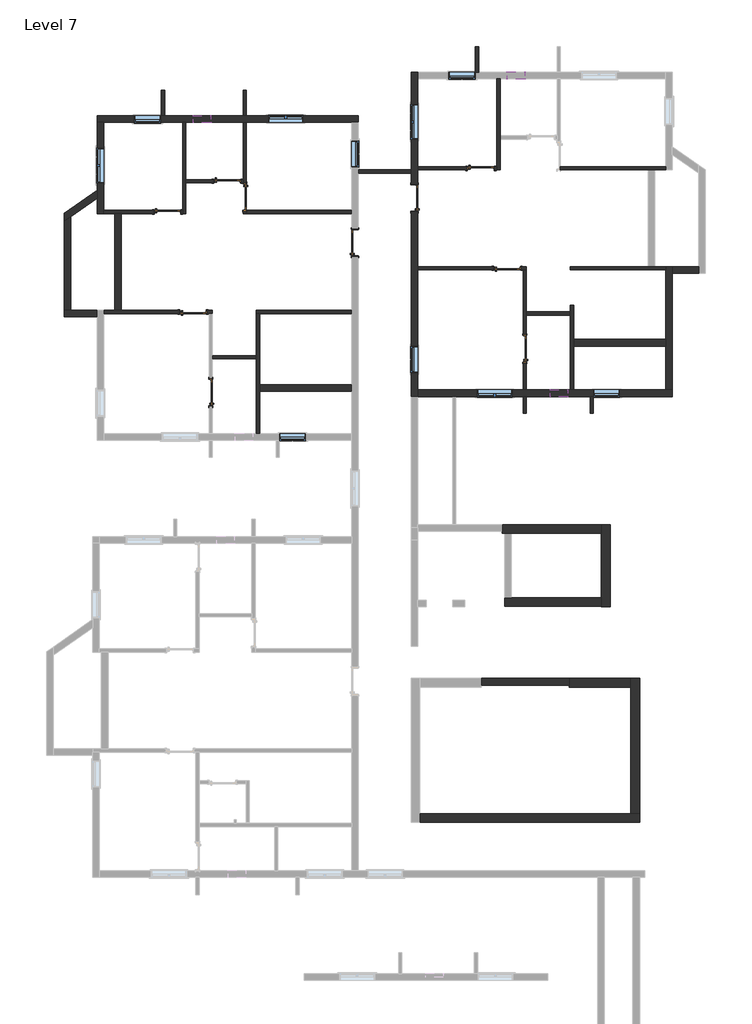
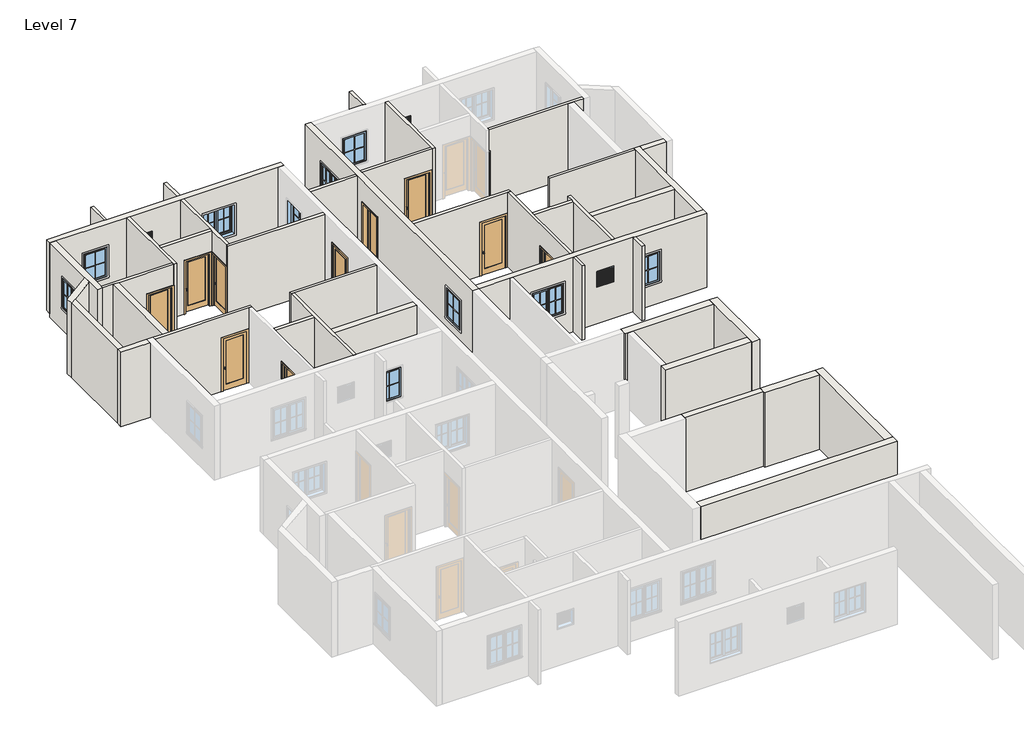
# One storey, part 5 of 7: 42 walls, 13 windows, 10 doors.
"""IFC4 building model written with IfcOpenShell, lengths in millimetres."""

from ifc_helpers import new_model, si_unit, frame, origin, place, context, project, spatial, polyline, outline, extrude, faceted_brep, transform, mapped, element, save
from components import door_3c6ab76a, door_a3feeac7, door_3b97b8e7, door_868ee8a9, window_272f20d6, window_casement_double_4_x_4_af3140d2, window_f2d8fef0

model = new_model("IFC4")

# Units and contexts
model_context = context("Model", 3, world=origin())
ifc_project = project(units=[si_unit("LENGTHUNIT", "METRE", prefix="MILLI")], contexts=[model_context])

# Site, building, storey
site = spatial("IfcSite", under=ifc_project)
building = spatial("IfcBuilding", under=site)
storey = spatial("IfcBuildingStorey", under=building, Name="Level 7", Elevation=9601.2)

# Doors
placement = place(None, origin())
door_shape = door_3c6ab76a(model_context)
element("IfcDoor", 1, ObjectType="Door-Interior-Single-1_Panel-Wood : 2'6\" x 7' door", at=placement, inside=storey, context=model_context, shape_type="MappedRepresentation", body=[
    mapped(door_shape, transform((-10226.9509469, 25492.3711172, 9601.2), x_axis=(1.0, 0.0, 0.0), y_axis=(0.0, 1.0, 0.0), z_axis=(0.0, 0.0, 1.0))),
])
door_2_shape = door_a3feeac7(model_context)
element("IfcDoor", 2, ObjectType="Door-Interior-Single-1_Panel-Wood : 2'6\" x 7' door", at=placement, inside=storey, context=model_context, shape_type="MappedRepresentation", body=[
    mapped(door_2_shape, transform((-10795.2759469, 18161.2961172, 9601.2), x_axis=(0.0, 1.0, 0.0), y_axis=(-1.0, 0.0, 0.0), z_axis=(0.0, 0.0, 1.0))),
])
element("IfcDoor", 3, ObjectType="Door-Interior-Single-1_Panel-Wood : 2'6\" x 7' door", at=placement, inside=storey, context=model_context, shape_type="MappedRepresentation", body=[
    mapped(door_2_shape, transform((101.3240531, 19674.7755084, 9601.2), x_axis=(0.0, 1.0, 0.0), y_axis=(-1.0, 0.0, 0.0), z_axis=(0.0, 0.0, 1.0))),
])
element("IfcDoor", 4, ObjectType="Door-Interior-Single-1_Panel-Wood : 36\" x 84\"", at=placement, inside=storey, context=model_context, shape_type="MappedRepresentation", body=[
    mapped(door_shape, transform((-12297.0509469, 24425.5711172, 9601.2), x_axis=(1.0, 0.0, 0.0), y_axis=(0.0, 1.0, 0.0), z_axis=(0.0, 0.0, 1.0))),
])
element("IfcDoor", 5, ObjectType="Door-Interior-Single-1_Panel-Wood : 36\" x 84\"", at=placement, inside=storey, context=model_context, shape_type="MappedRepresentation", body=[
    mapped(door_shape, transform((-9614.1759469, 24936.7461172, 9601.2), x_axis=(0.0, -1.0, 0.0), y_axis=(1.0, 0.0, 0.0), z_axis=(0.0, 0.0, 1.0))),
])
element("IfcDoor", 6, ObjectType="Door-Interior-Single-1_Panel-Wood : 36\" x 84\"", at=placement, inside=storey, context=model_context, shape_type="MappedRepresentation", body=[
    mapped(door_shape, transform((-1425.8509469, 25939.0505084, 9601.2), x_axis=(1.0, 0.0, 0.0), y_axis=(0.0, 1.0, 0.0), z_axis=(0.0, 0.0, 1.0))),
])
door_3_shape = door_3b97b8e7(model_context)
element("IfcDoor", 7, ObjectType="Door-Interior-Single-1_Panel-Wood : 36\" x 84\"", at=placement, inside=storey, context=model_context, shape_type="MappedRepresentation", body=[
    mapped(door_3_shape, transform((-5791.4759469, 23355.5961172, 9601.2), x_axis=(0.0, 1.0, 0.0), y_axis=(-1.0, 0.0, 0.0), z_axis=(0.0, 0.0, 1.0))),
])
element("IfcDoor", 8, ObjectType="Door-Interior-Single-1_Panel-Wood : 36\" x 84\"", at=placement, inside=storey, context=model_context, shape_type="MappedRepresentation", body=[
    mapped(door_2_shape, transform((-11408.0509469, 20952.1211172, 9601.2), x_axis=(1.0, 0.0, 0.0), y_axis=(0.0, 1.0, 0.0), z_axis=(0.0, 0.0, 1.0))),
])
element("IfcDoor", 9, ObjectType="Door-Interior-Single-1_Panel-Wood : 36\" x 84\"", at=placement, inside=storey, context=model_context, shape_type="MappedRepresentation", body=[
    mapped(door_2_shape, transform((-511.4509469, 22465.6005084, 9601.2), x_axis=(1.0, 0.0, 0.0), y_axis=(0.0, 1.0, 0.0), z_axis=(0.0, 0.0, 1.0))),
])
door_4_shape = door_868ee8a9(model_context)
element("IfcDoor", 10, ObjectType="Door-Interior-Single-1_Panel-Wood : 36\" x 84\"", at=placement, inside=storey, context=model_context, shape_type="MappedRepresentation", body=[
    mapped(door_4_shape, transform((-3727.7259469, 24907.1755084, 9601.2), x_axis=(0.0, 1.0, 0.0), y_axis=(-1.0, 0.0, 0.0), z_axis=(0.0, 0.0, 1.0))),
])

# Walls
element("IfcWall", 11, ObjectType="1' feet", at=placement, inside=storey, context=model_context, shape_type="Brep", body=[
    faceted_brep([(-682.9009469, 13266.6182723, 9601.2), (2758.7990531, 13266.6182723, 9601.2), (2758.7990531, 13266.6182723, 12649.2), (-682.9009469, 13266.6182723, 12649.2), (-682.9009469, 13571.4182723, 9601.2), (-682.9009469, 13571.4182723, 12649.2), (2758.7990531, 13571.4182723, 12649.2), (2758.7990531, 13571.4182723, 9601.2), (-682.9009469, 13342.8182723, 9601.2), (-682.9009469, 13342.8182723, 12649.2)], [[[0, 1, 2, 3]], [[4, 5, 6, 7]], [[1, 0, 8, 4, 7]], [[3, 2, 6, 5, 9]], [[0, 3, 9, 5, 4, 8]], [[2, 1, 7, 6]]]),
])
element("IfcWall", 12, ObjectType="1' feet", at=placement, inside=storey, context=model_context, shape_type="Brep", body=[
    faceted_brep([(3063.5990531, 10726.6182723, 9601.2), (3063.5990531, 13571.4182723, 9601.2), (3063.5990531, 13571.4182723, 12649.2), (3063.5990531, 10726.6182723, 12649.2), (2758.7990531, 10726.6182723, 9601.2), (2758.7990531, 10726.6182723, 12649.2), (2758.7990531, 10739.3182723, 12649.2), (2758.7990531, 11044.1182723, 12649.2), (2758.7990531, 13266.6182723, 12649.2), (2758.7990531, 13571.4182723, 12649.2), (2758.7990531, 13571.4182723, 9601.2), (2758.7990531, 13266.6182723, 9601.2), (2758.7990531, 11044.1182723, 9601.2), (2758.7990531, 10739.3182723, 9601.2)], [[[0, 1, 2, 3]], [[4, 5, 6, 7, 8, 9, 10, 11, 12, 13]], [[1, 0, 4, 13, 12, 11, 10]], [[3, 2, 9, 8, 7, 6, 5]], [[0, 3, 5, 4]], [[2, 1, 10, 9]]]),
])
element("IfcWall", 13, ObjectType="1' feet", at=placement, inside=storey, context=model_context, shape_type="Brep", body=[
    faceted_brep([(2758.7990531, 11044.1182723, 9601.2), (-365.4009469, 11044.1182723, 9601.2), (-594.0009469, 11044.1182723, 9601.2), (-594.0009469, 11044.1182723, 12649.2), (-365.4009469, 11044.1182723, 12649.2), (2758.7990531, 11044.1182723, 12649.2), (2758.7990531, 10739.3182723, 9601.2), (2758.7990531, 10739.3182723, 12649.2), (-594.0009469, 10739.3182723, 12649.2), (-594.0009469, 10739.3182723, 9601.2)], [[[0, 1, 2, 3, 4, 5]], [[6, 7, 8, 9]], [[2, 1, 0, 6, 9]], [[5, 4, 3, 8, 7]], [[0, 5, 7, 6]], [[3, 2, 9, 8]]]),
])
element("IfcWall", 14, ObjectType="1' feet", at=placement, inside=storey, context=model_context, shape_type="Brep", body=[
    faceted_brep([(-3540.4009469, 3245.1461172, 9601.2), (4079.5990531, 3245.1461172, 9601.2), (4079.5990531, 3245.1461172, 12649.2), (-3540.4009469, 3245.1461172, 12649.2), (-3540.4009469, 3549.9461172, 9601.2), (-3540.4009469, 3549.9461172, 12649.2), (3774.7990531, 3549.9461172, 12649.2), (4079.5990531, 3549.9461172, 12649.2), (4079.5990531, 3549.9461172, 9601.2), (3774.7990531, 3549.9461172, 9601.2)], [[[0, 1, 2, 3]], [[4, 5, 6, 7, 8, 9]], [[1, 0, 4, 9, 8]], [[3, 2, 7, 6, 5]], [[2, 1, 8, 7]], [[0, 3, 5, 4]]]),
])
element("IfcWall", 15, ObjectType="1' feet", at=placement, inside=storey, context=model_context, shape_type="Brep", body=[
    faceted_brep([(4079.5990531, 3549.9461172, 9601.2), (4079.5990531, 8236.2461172, 9601.2), (4079.5990531, 8236.2461172, 12649.2), (4079.5990531, 3549.9461172, 12649.2), (3774.7990531, 3549.9461172, 9601.2), (3774.7990531, 3549.9461172, 12649.2), (3774.7990531, 7931.4461172, 12649.2), (3774.7990531, 8236.2461172, 12649.2), (3774.7990531, 8236.2461172, 9601.2), (3774.7990531, 7931.4461172, 9601.2)], [[[0, 1, 2, 3]], [[4, 5, 6, 7, 8, 9]], [[1, 0, 4, 9, 8]], [[3, 2, 7, 6, 5]], [[0, 3, 5, 4]], [[2, 1, 8, 7]]]),
])
element("IfcWall", 16, ObjectType="1' feet", at=placement, inside=storey, context=model_context, shape_type="Brep", body=[
    faceted_brep([(1641.1990531, 7931.4461172, 9601.2), (3774.7990531, 7931.4461172, 9601.2), (3774.7990531, 7931.4461172, 12649.2), (1641.1990531, 7931.4461172, 12649.2), (1641.1990531, 8236.2461172, 9601.2), (1641.1990531, 8236.2461172, 12649.2), (3774.7990531, 8236.2461172, 12649.2), (3774.7990531, 8236.2461172, 9601.2), (1641.1990531, 8007.6461172, 9601.2), (1641.1990531, 8007.6461172, 12649.2)], [[[0, 1, 2, 3]], [[4, 5, 6, 7]], [[1, 0, 8, 4, 7]], [[3, 2, 6, 5, 9]], [[0, 3, 9, 5, 4, 8]], [[2, 1, 7, 6]]]),
])
element("IfcWall", 17, ObjectType="4.5\" wall", at=placement, inside=storey, context=model_context, shape_type="Brep", body=[
    faceted_brep([(-11655.7009469, 24365.2461172, 9601.2), (-11655.7009469, 25432.0461172, 9601.2), (-11655.7009469, 25546.3461172, 9601.2), (-11655.7009469, 27527.5461172, 9601.2), (-11655.7009469, 27527.5461172, 12649.2), (-11655.7009469, 25546.3461172, 12649.2), (-11655.7009469, 25432.0461172, 12649.2), (-11655.7009469, 24365.2461172, 12649.2), (-11770.0009469, 24365.2461172, 9601.2), (-11770.0009469, 24365.2461172, 12649.2), (-11770.0009469, 24479.5461172, 12649.2), (-11770.0009469, 27527.5461172, 12649.2), (-11770.0009469, 27527.5461172, 9601.2), (-11770.0009469, 24479.5461172, 9601.2)], [[[0, 1, 2, 3, 4, 5, 6, 7]], [[8, 9, 10, 11, 12, 13]], [[3, 2, 1, 0, 8, 13, 12]], [[7, 6, 5, 4, 11, 10, 9]], [[4, 3, 12, 11]], [[0, 7, 9, 8]]]),
])
element("IfcWall", 18, ObjectType="4.5\" wall", at=placement, inside=storey, context=model_context, shape_type="SweptSolid", body=[
    extrude(outline(polyline([(12649.2, -9674.5009469), (12649.2, -11655.7009469), (9601.2, -11655.7009469), (9601.2, -10709.5509469), (11760.2, -10709.5509469), (11760.2, -9744.3509469), (9601.2, -9744.3509469), (9601.2, -9674.5009469), (12649.2, -9674.5009469)])), frame((0.0, 25432.0461172, 0.0), z_axis=(0.0, 1.0, 0.0), x_axis=(0.0, 0.0, 1.0)), (0.0, 0.0, 1.0), 114.3),
])
element("IfcWall", 19, ObjectType="4.5\" wall", at=placement, inside=storey, context=model_context, shape_type="Brep", body=[
    faceted_brep([(-11770.0009469, 24365.2461172, 12649.2), (-13903.6009469, 24365.2461172, 12649.2), (-14132.2009469, 24365.2461172, 12649.2), (-14513.2009469, 24365.2461172, 12649.2), (-14513.2009469, 24365.2461172, 9601.2), (-14132.2009469, 24365.2461172, 9601.2), (-13903.6009469, 24365.2461172, 9601.2), (-12779.6509469, 24365.2461172, 9601.2), (-12779.6509469, 24365.2461172, 11760.2), (-11814.4509469, 24365.2461172, 11760.2), (-11814.4509469, 24365.2461172, 9601.2), (-11770.0009469, 24365.2461172, 9601.2), (-14513.2009469, 24479.5461172, 12649.2), (-11770.0009469, 24479.5461172, 12649.2), (-11770.0009469, 24479.5461172, 9601.2), (-11814.4509469, 24479.5461172, 9601.2), (-11814.4509469, 24479.5461172, 11760.2), (-12779.6509469, 24479.5461172, 11760.2), (-12779.6509469, 24479.5461172, 9601.2), (-14513.2009469, 24479.5461172, 9601.2)], [[[0, 1, 2, 3, 4, 5, 6, 7, 8, 9, 10, 11]], [[12, 13, 14, 15, 16, 17, 18, 19]], [[4, 19, 18, 7, 6, 5]], [[14, 11, 10, 15]], [[3, 2, 1, 0, 13, 12]], [[4, 3, 12, 19]], [[0, 11, 14, 13]], [[9, 16, 15, 10]], [[16, 9, 8, 17]], [[17, 8, 7, 18]]]),
])
element("IfcWall", 20, ObjectType="4.5\" wall", at=placement, inside=storey, context=model_context, shape_type="Brep", body=[
    faceted_brep([(-9674.5009469, 24479.5461172, 12649.2), (-9560.2009469, 24479.5461172, 12649.2), (-5902.6009469, 24479.5461172, 12649.2), (-5902.6009469, 24479.5461172, 9601.2), (-9560.2009469, 24479.5461172, 9601.2), (-9560.2009469, 24479.5461172, 11760.2), (-9674.5009469, 24479.5461172, 11760.2), (-9674.5009469, 24365.2461172, 9601.2), (-5902.6009469, 24365.2461172, 9601.2), (-5902.6009469, 24365.2461172, 12649.2), (-9674.5009469, 24365.2461172, 12649.2), (-9674.5009469, 24454.1461172, 9601.2), (-9560.2009469, 24454.1461172, 9601.2), (-9674.5009469, 24454.1461172, 11760.2), (-9560.2009469, 24454.1461172, 11760.2)], [[[0, 1, 2, 3, 4, 5, 6]], [[7, 8, 9, 10]], [[8, 7, 11, 12, 4, 3]], [[2, 1, 0, 10, 9]], [[7, 10, 0, 6, 13, 11]], [[3, 2, 9, 8]], [[12, 14, 5, 4]], [[14, 12, 11, 13]], [[14, 13, 6, 5]]]),
])
element("IfcWall", 21, ObjectType="4.5\" wall", at=placement, inside=storey, context=model_context, shape_type="Brep", body=[
    faceted_brep([(-5902.6009469, 21012.4461172, 9601.2), (-9217.3009469, 21012.4461172, 9601.2), (-9217.3009469, 21012.4461172, 12649.2), (-5902.6009469, 21012.4461172, 12649.2), (-5902.6009469, 20898.1461172, 9601.2), (-5902.6009469, 20898.1461172, 12649.2), (-9103.0009469, 20898.1461172, 12649.2), (-9217.3009469, 20898.1461172, 12649.2), (-9217.3009469, 20898.1461172, 9601.2), (-9103.0009469, 20898.1461172, 9601.2)], [[[0, 1, 2, 3]], [[4, 5, 6, 7, 8, 9]], [[1, 0, 4, 9, 8]], [[3, 2, 7, 6, 5]], [[0, 3, 5, 4]], [[2, 1, 8, 7]]]),
])
element("IfcWall", 22, ObjectType="4.5\" wall", at=placement, inside=storey, context=model_context, shape_type="Brep", body=[
    faceted_brep([(-14513.2009469, 21012.4461172, 12649.2), (-14132.2009469, 21012.4461172, 12649.2), (-13903.6009469, 21012.4461172, 12649.2), (-10741.3009469, 21012.4461172, 12649.2), (-10741.3009469, 21012.4461172, 9601.2), (-10925.4509469, 21012.4461172, 9601.2), (-10925.4509469, 21012.4461172, 11760.2), (-11890.6509469, 21012.4461172, 11760.2), (-11890.6509469, 21012.4461172, 9601.2), (-13903.6009469, 21012.4461172, 9601.2), (-14132.2009469, 21012.4461172, 9601.2), (-14513.2009469, 21012.4461172, 9601.2), (-10741.3009469, 20898.1461172, 12649.2), (-10855.6009469, 20898.1461172, 12649.2), (-14513.2009469, 20898.1461172, 12649.2), (-14513.2009469, 20898.1461172, 9601.2), (-11890.6509469, 20898.1461172, 9601.2), (-11890.6509469, 20898.1461172, 11760.2), (-10925.4509469, 20898.1461172, 11760.2), (-10925.4509469, 20898.1461172, 9601.2), (-10855.6009469, 20898.1461172, 9601.2), (-10741.3009469, 20898.1461172, 9601.2)], [[[0, 1, 2, 3, 4, 5, 6, 7, 8, 9, 10, 11]], [[12, 13, 14, 15, 16, 17, 18, 19, 20, 21]], [[15, 11, 10, 9, 8, 16]], [[4, 21, 20, 19, 5]], [[3, 2, 1, 0, 14, 13, 12]], [[0, 11, 15, 14]], [[4, 3, 12, 21]], [[18, 6, 5, 19]], [[6, 18, 17, 7]], [[7, 17, 16, 8]]]),
])
element("IfcWall", 23, ObjectType="4.5\" wall", at=placement, inside=storey, context=model_context, shape_type="Brep", body=[
    faceted_brep([(-9560.2009469, 27527.5461172, 12649.2), (-9560.2009469, 24479.5461172, 12649.2), (-9560.2009469, 24479.5461172, 11760.2), (-9560.2009469, 25419.3461172, 11760.2), (-9560.2009469, 25419.3461172, 9601.2), (-9560.2009469, 27527.5461172, 9601.2), (-9674.5009469, 24479.5461172, 12649.2), (-9674.5009469, 25432.0461172, 12649.2), (-9674.5009469, 25546.3461172, 12649.2), (-9674.5009469, 27527.5461172, 12649.2), (-9674.5009469, 27527.5461172, 9601.2), (-9674.5009469, 25546.3461172, 9601.2), (-9674.5009469, 25432.0461172, 9601.2), (-9674.5009469, 25419.3461172, 9601.2), (-9674.5009469, 25419.3461172, 11760.2), (-9674.5009469, 24479.5461172, 11760.2)], [[[0, 1, 2, 3, 4, 5]], [[6, 7, 8, 9, 10, 11, 12, 13, 14, 15]], [[10, 5, 4, 13, 12, 11]], [[1, 0, 9, 8, 7, 6]], [[0, 5, 10, 9]], [[1, 6, 15, 2]], [[14, 3, 2, 15]], [[3, 14, 13, 4]]]),
])
element("IfcWall", 24, ObjectType="4.5\" wall", at=placement, inside=storey, context=model_context, shape_type="SweptSolid", body=[
    extrude(outline(polyline([(-9217.3009469, 19323.3461172), (-10741.3009469, 19323.3461172), (-10741.3009469, 19437.6461172), (-9217.3009469, 19437.6461172), (-9217.3009469, 19323.3461172)])), frame((0.0, 0.0, 9601.2), z_axis=(0.0, 0.0, 1.0), x_axis=(1.0, 0.0, 0.0)), (0.0, 0.0, 1.0), 3048.0),
])
element("IfcWall", 25, ObjectType="4.5\" wall", at=placement, inside=storey, context=model_context, shape_type="Brep", body=[
    faceted_brep([(-9217.3009469, 20898.1461172, 9601.2), (-9217.3009469, 19437.6461172, 9601.2), (-9217.3009469, 19323.3461172, 9601.2), (-9217.3009469, 16732.5461172, 9601.2), (-9217.3009469, 16732.5461172, 12649.2), (-9217.3009469, 19323.3461172, 12649.2), (-9217.3009469, 19437.6461172, 12649.2), (-9217.3009469, 20898.1461172, 12649.2), (-9103.0009469, 20898.1461172, 9601.2), (-9103.0009469, 20898.1461172, 12649.2), (-9103.0009469, 18434.3461172, 12649.2), (-9103.0009469, 18205.7461172, 12649.2), (-9103.0009469, 16732.5461172, 12649.2), (-9103.0009469, 16732.5461172, 9601.2), (-9103.0009469, 18205.7461172, 9601.2), (-9103.0009469, 18434.3461172, 9601.2)], [[[0, 1, 2, 3, 4, 5, 6, 7]], [[8, 9, 10, 11, 12, 13, 14, 15]], [[3, 2, 1, 0, 8, 15, 14, 13]], [[7, 6, 5, 4, 12, 11, 10, 9]], [[0, 7, 9, 8]], [[4, 3, 13, 12]]]),
])
element("IfcWall", 26, ObjectType="4.5\" wall", at=placement, inside=storey, context=model_context, shape_type="SweptSolid", body=[
    extrude(outline(polyline([(-5674.0009469, 25878.7255084), (-3845.2009469, 25878.7255084), (-3845.2009469, 25764.4255084), (-5674.0009469, 25764.4255084), (-5674.0009469, 25878.7255084)])), frame((0.0, 0.0, 9601.2), z_axis=(0.0, 0.0, 1.0), x_axis=(1.0, 0.0, 0.0)), (0.0, 0.0, 1.0), 3048.0),
])
element("IfcWall", 27, ObjectType="4.5\" wall", at=placement, inside=storey, context=model_context, shape_type="Brep", body=[
    faceted_brep([(-759.1009469, 25878.7255084, 9601.2), (-759.1009469, 26945.5255084, 9601.2), (-759.1009469, 27059.8255084, 9601.2), (-759.1009469, 29041.0255084, 9601.2), (-759.1009469, 29041.0255084, 12649.2), (-759.1009469, 27059.8255084, 12649.2), (-759.1009469, 26945.5255084, 12649.2), (-759.1009469, 25878.7255084, 12649.2), (-873.4009469, 25878.7255084, 9601.2), (-873.4009469, 25878.7255084, 12649.2), (-873.4009469, 25993.0255084, 12649.2), (-873.4009469, 29041.0255084, 12649.2), (-873.4009469, 29041.0255084, 9601.2), (-873.4009469, 25993.0255084, 9601.2)], [[[0, 1, 2, 3, 4, 5, 6, 7]], [[8, 9, 10, 11, 12, 13]], [[3, 2, 1, 0, 8, 13, 12]], [[7, 6, 5, 4, 11, 10, 9]], [[4, 3, 12, 11]], [[0, 7, 9, 8]]]),
])
element("IfcWall", 28, ObjectType="4.5\" wall", at=placement, inside=storey, context=model_context, shape_type="SweptSolid", body=[
    extrude(outline(polyline([(12649.2, -873.4009469), (12649.2, -3616.6009469), (9601.2, -3616.6009469), (9601.2, -1908.4509469), (11760.2, -1908.4509469), (11760.2, -943.2509469), (9601.2, -943.2509469), (9601.2, -873.4009469), (12649.2, -873.4009469)])), frame((0.0, 25878.7255084, 0.0), z_axis=(0.0, 1.0, 0.0), x_axis=(0.0, 0.0, 1.0)), (0.0, 0.0, 1.0), 114.3),
])
element("IfcWall", 29, ObjectType="4.5\" wall", at=placement, inside=storey, context=model_context, shape_type="Brep", body=[
    faceted_brep([(4993.9990531, 25993.0255084, 9601.2), (1336.3990531, 25993.0255084, 9601.2), (1336.3990531, 25993.0255084, 12649.2), (4993.9990531, 25993.0255084, 12649.2), (4993.9990531, 25878.7255084, 9601.2), (4993.9990531, 25878.7255084, 12649.2), (4612.9990531, 25878.7255084, 12649.2), (4384.3990531, 25878.7255084, 12649.2), (1336.3990531, 25878.7255084, 12649.2), (1336.3990531, 25878.7255084, 9601.2), (4384.3990531, 25878.7255084, 9601.2), (4612.9990531, 25878.7255084, 9601.2)], [[[0, 1, 2, 3]], [[4, 5, 6, 7, 8, 9, 10, 11]], [[1, 0, 4, 11, 10, 9]], [[3, 2, 8, 7, 6, 5]], [[2, 1, 9, 8]], [[0, 3, 5, 4]]]),
])
element("IfcWall", 30, ObjectType="4.5\" wall", at=placement, inside=storey, context=model_context, shape_type="Brep", body=[
    faceted_brep([(4993.9990531, 22525.9255084, 9601.2), (4612.9990531, 22525.9255084, 9601.2), (4384.3990531, 22525.9255084, 9601.2), (1679.2990531, 22525.9255084, 9601.2), (1679.2990531, 22525.9255084, 12649.2), (4384.3990531, 22525.9255084, 12649.2), (4612.9990531, 22525.9255084, 12649.2), (4993.9990531, 22525.9255084, 12649.2), (4993.9990531, 22411.6255084, 9601.2), (4993.9990531, 22411.6255084, 12649.2), (1679.2990531, 22411.6255084, 12649.2), (1679.2990531, 22411.6255084, 9601.2)], [[[0, 1, 2, 3, 4, 5, 6, 7]], [[8, 9, 10, 11]], [[3, 2, 1, 0, 8, 11]], [[4, 3, 11, 10]], [[7, 6, 5, 4, 10, 9]], [[0, 7, 9, 8]]]),
])
element("IfcWall", 31, ObjectType="4.5\" wall", at=placement, inside=storey, context=model_context, shape_type="Brep", body=[
    faceted_brep([(155.2990531, 22411.6255084, 12649.2), (40.9990531, 22411.6255084, 12649.2), (-3616.6009469, 22411.6255084, 12649.2), (-3616.6009469, 22411.6255084, 9601.2), (-994.0509469, 22411.6255084, 9601.2), (-994.0509469, 22411.6255084, 11760.2), (-28.8509469, 22411.6255084, 11760.2), (-28.8509469, 22411.6255084, 9601.2), (40.9990531, 22411.6255084, 9601.2), (155.2990531, 22411.6255084, 9601.2), (-3616.6009469, 22525.9255084, 12649.2), (155.2990531, 22525.9255084, 12649.2), (155.2990531, 22525.9255084, 9601.2), (-28.8509469, 22525.9255084, 9601.2), (-28.8509469, 22525.9255084, 11760.2), (-994.0509469, 22525.9255084, 11760.2), (-994.0509469, 22525.9255084, 9601.2), (-3616.6009469, 22525.9255084, 9601.2)], [[[0, 1, 2, 3, 4, 5, 6, 7, 8, 9]], [[10, 11, 12, 13, 14, 15, 16, 17]], [[3, 17, 16, 4]], [[12, 9, 8, 7, 13]], [[2, 1, 0, 11, 10]], [[3, 2, 10, 17]], [[0, 9, 12, 11]], [[6, 14, 13, 7]], [[14, 6, 5, 15]], [[15, 5, 4, 16]]]),
])
element("IfcWall", 32, ObjectType="4.5\" wall", at=placement, inside=storey, context=model_context, shape_type="Brep", body=[
    faceted_brep([(155.2990531, 22411.6255084, 12649.2), (155.2990531, 20951.1255084, 12649.2), (155.2990531, 20836.8255084, 12649.2), (155.2990531, 18246.0255084, 12649.2), (155.2990531, 18246.0255084, 9601.2), (155.2990531, 19192.1755084, 9601.2), (155.2990531, 19192.1755084, 11760.2), (155.2990531, 20157.3755084, 11760.2), (155.2990531, 20157.3755084, 9601.2), (155.2990531, 20836.8255084, 9601.2), (155.2990531, 20951.1255084, 9601.2), (155.2990531, 22411.6255084, 9601.2), (40.9990531, 18246.0255084, 12649.2), (40.9990531, 22411.6255084, 12649.2), (40.9990531, 22411.6255084, 9601.2), (40.9990531, 20157.3755084, 9601.2), (40.9990531, 20157.3755084, 11760.2), (40.9990531, 19192.1755084, 11760.2), (40.9990531, 19192.1755084, 9601.2), (40.9990531, 18246.0255084, 9601.2)], [[[0, 1, 2, 3, 4, 5, 6, 7, 8, 9, 10, 11]], [[12, 13, 14, 15, 16, 17, 18, 19]], [[14, 11, 10, 9, 8, 15]], [[4, 19, 18, 5]], [[3, 2, 1, 0, 13, 12]], [[0, 11, 14, 13]], [[4, 3, 12, 19]], [[7, 16, 15, 8]], [[16, 7, 6, 17]], [[17, 6, 5, 18]]]),
])
element("IfcWall", 33, ObjectType="4.5\" wall", at=placement, inside=storey, context=model_context, shape_type="Brep", body=[
    faceted_brep([(1679.2990531, 21192.4255084, 9601.2), (1679.2990531, 20951.1255084, 9601.2), (1679.2990531, 20836.8255084, 9601.2), (1679.2990531, 18246.0255084, 9601.2), (1679.2990531, 18246.0255084, 12649.2), (1679.2990531, 20836.8255084, 12649.2), (1679.2990531, 20951.1255084, 12649.2), (1679.2990531, 21192.4255084, 12649.2), (1793.5990531, 21192.4255084, 9601.2), (1793.5990531, 21192.4255084, 12649.2), (1793.5990531, 19998.6255084, 12649.2), (1793.5990531, 19770.0255084, 12649.2), (1793.5990531, 18246.0255084, 12649.2), (1793.5990531, 18246.0255084, 9601.2), (1793.5990531, 19770.0255084, 9601.2), (1793.5990531, 19998.6255084, 9601.2)], [[[0, 1, 2, 3, 4, 5, 6, 7]], [[8, 9, 10, 11, 12, 13, 14, 15]], [[3, 2, 1, 0, 8, 15, 14, 13]], [[7, 6, 5, 4, 12, 11, 10, 9]], [[0, 7, 9, 8]], [[4, 3, 13, 12]]]),
])
element("IfcWall", 34, ObjectType="4.5\" wall", at=placement, inside=storey, context=model_context, shape_type="SweptSolid", body=[
    extrude(outline(polyline([(155.2990531, 20951.1255084), (1679.2990531, 20951.1255084), (1679.2990531, 20836.8255084), (155.2990531, 20836.8255084), (155.2990531, 20951.1255084)])), frame((0.0, 0.0, 9601.2), z_axis=(0.0, 0.0, 1.0), x_axis=(1.0, 0.0, 0.0)), (0.0, 0.0, 1.0), 3048.0),
])
element("IfcWall", 35, ObjectType="4.5\" wall", at=placement, inside=storey, context=model_context, shape_type="Brep", body=[
    faceted_brep([(-1617.8862554, 30161.6889788, 9601.2), (-1617.8862554, 29269.6255084, 9601.2), (-1617.8862554, 29269.6255084, 10515.6), (-1617.8862554, 29269.6255084, 11734.8), (-1617.8862554, 29269.6255084, 12649.2), (-1617.8862554, 30161.6889788, 12649.2), (-1503.5862554, 30161.6889788, 9601.2), (-1503.5862554, 30161.6889788, 12649.2), (-1503.5862554, 29269.6255084, 12649.2), (-1503.5862554, 29269.6255084, 9601.2)], [[[0, 1, 2, 3, 4, 5]], [[6, 7, 8, 9]], [[1, 0, 6, 9]], [[5, 4, 8, 7]], [[0, 5, 7, 6]], [[4, 3, 2, 1, 9, 8]]]),
])
element("IfcWall", 36, ObjectType="4.5\" wall", at=placement, inside=storey, context=model_context, shape_type="SweptSolid", body=[
    extrude(outline(polyline([(40.9990531, 17431.8689406), (40.9990531, 18017.4255084), (155.2990531, 18017.4255084), (155.2990531, 17431.8689406), (40.9990531, 17431.8689406)])), frame((0.0, 0.0, 9601.2), z_axis=(0.0, 0.0, 1.0), x_axis=(1.0, 0.0, 0.0)), (0.0, 0.0, 1.0), 3048.0),
])
element("IfcWall", 37, ObjectType="4.5\" wall", at=placement, inside=storey, context=model_context, shape_type="Brep", body=[
    faceted_brep([(2365.0990531, 18017.4255084, 9601.2), (2365.0990531, 17431.8689406, 9601.2), (2365.0990531, 17431.8689406, 12649.2), (2365.0990531, 18017.4255084, 12649.2), (2479.3990531, 18017.4255084, 9601.2), (2479.3990531, 18017.4255084, 10515.6), (2479.3990531, 18017.4255084, 11734.8), (2479.3990531, 18017.4255084, 12649.2), (2479.3990531, 17431.8689406, 12649.2), (2479.3990531, 17431.8689406, 9601.2)], [[[0, 1, 2, 3]], [[4, 5, 6, 7, 8, 9]], [[1, 0, 4, 9]], [[2, 1, 9, 8]], [[3, 2, 8, 7]], [[0, 3, 7, 6, 5, 4]]]),
])
element("IfcWall", 38, ObjectType="4.5\" wall", at=placement, inside=storey, context=model_context, shape_type="SweptSolid", body=[
    extrude(outline(polyline([(-12514.4862554, 27756.1461172), (-12514.4862554, 28648.2095876), (-12400.1862554, 28648.2095876), (-12400.1862554, 27756.1461172), (-12514.4862554, 27756.1461172)])), frame((0.0, 0.0, 9601.2), z_axis=(0.0, 0.0, 1.0), x_axis=(1.0, 0.0, 0.0)), (0.0, 0.0, 1.0), 3048.0),
])
element("IfcWall", 39, ObjectType="4.5\" wall", at=placement, inside=storey, context=model_context, shape_type="SweptSolid", body=[
    extrude(outline(polyline([(-9560.2009469, 28648.2095876), (-9560.2009469, 27756.1461172), (-9674.5009469, 27756.1461172), (-9674.5009469, 28648.2095876), (-9560.2009469, 28648.2095876)])), frame((0.0, 0.0, 9601.2), z_axis=(0.0, 0.0, 1.0), x_axis=(1.0, 0.0, 0.0)), (0.0, 0.0, 1.0), 3048.0),
])
element("IfcWall", 40, ObjectType="9\"", at=placement, inside=storey, context=model_context, shape_type="Brep", body=[
    faceted_brep([(-5674.0009469, 27756.1461172, 9753.6), (-14741.8009469, 27756.1461172, 9753.6), (-14741.8009469, 27756.1461172, 12649.2), (-12514.4862554, 27756.1461172, 12649.2), (-12400.1862554, 27756.1461172, 12649.2), (-9674.5009469, 27756.1461172, 12649.2), (-9560.2009469, 27756.1461172, 12649.2), (-5674.0009469, 27756.1461172, 12649.2), (-10798.4509469, 27756.1461172, 11734.8), (-11408.0509469, 27756.1461172, 11734.8), (-11408.0509469, 27756.1461172, 11125.2), (-10798.4509469, 27756.1461172, 11125.2), (-13447.9362554, 27756.1461172, 11734.8), (-13447.9362554, 27756.1461172, 10515.6), (-12533.5362554, 27756.1461172, 10515.6), (-12533.5362554, 27756.1461172, 11734.8), (-7585.3509469, 27756.1461172, 11734.8), (-8804.5509469, 27756.1461172, 11734.8), (-8804.5509469, 27756.1461172, 10515.6), (-7585.3509469, 27756.1461172, 10515.6), (-5674.0009469, 27527.5461172, 9753.6), (-5674.0009469, 27527.5461172, 12649.2), (-5902.6009469, 27527.5461172, 12649.2), (-9560.2009469, 27527.5461172, 12649.2), (-9674.5009469, 27527.5461172, 12649.2), (-11655.7009469, 27527.5461172, 12649.2), (-11770.0009469, 27527.5461172, 12649.2), (-14513.2009469, 27527.5461172, 12649.2), (-14741.8009469, 27527.5461172, 12649.2), (-14741.8009469, 27527.5461172, 9753.6), (-10798.4509469, 27527.5461172, 11734.8), (-10798.4509469, 27527.5461172, 11125.2), (-11408.0509469, 27527.5461172, 11125.2), (-11408.0509469, 27527.5461172, 11734.8), (-13447.9362554, 27527.5461172, 11734.8), (-12533.5362554, 27527.5461172, 11734.8), (-12533.5362554, 27527.5461172, 10515.6), (-13447.9362554, 27527.5461172, 10515.6), (-7585.3509469, 27527.5461172, 11734.8), (-7585.3509469, 27527.5461172, 10515.6), (-8804.5509469, 27527.5461172, 10515.6), (-8804.5509469, 27527.5461172, 11734.8)], [[[0, 1, 2, 3, 4, 5, 6, 7], [8, 9, 10, 11], [12, 13, 14, 15], [16, 17, 18, 19]], [[20, 21, 22, 23, 24, 25, 26, 27, 28, 29], [30, 31, 32, 33], [34, 35, 36, 37], [38, 39, 40, 41]], [[1, 0, 20, 29]], [[7, 6, 5, 4, 3, 2, 28, 27, 26, 25, 24, 23, 22, 21]], [[2, 1, 29, 28]], [[0, 7, 21, 20]], [[31, 30, 8, 11]], [[32, 31, 11, 10]], [[33, 32, 10, 9]], [[30, 33, 9, 8]], [[13, 12, 34, 37]], [[14, 13, 37, 36]], [[15, 14, 36, 35]], [[12, 15, 35, 34]], [[39, 38, 16, 19]], [[40, 39, 19, 18]], [[41, 40, 18, 17]], [[38, 41, 17, 16]]]),
])
element("IfcWall", 41, ObjectType="9\"", at=placement, inside=storey, context=model_context, shape_type="Brep", body=[
    faceted_brep([(-14741.8009469, 27527.5461172, 9601.2), (-14741.8009469, 25177.6879786, 9601.2), (-14741.8009469, 24898.6461172, 9601.2), (-14741.8009469, 24365.2461172, 9601.2), (-14741.8009469, 24365.2461172, 12649.2), (-14741.8009469, 24898.6461172, 12649.2), (-14741.8009469, 25177.6879786, 12649.2), (-14741.8009469, 27527.5461172, 12649.2), (-14741.8009469, 27527.5461172, 9753.6), (-14741.8009469, 26641.7211172, 11734.8), (-14741.8009469, 25422.5211172, 11734.8), (-14741.8009469, 25422.5211172, 10515.6), (-14741.8009469, 26641.7211172, 10515.6), (-14513.2009469, 27527.5461172, 9601.2), (-14513.2009469, 27527.5461172, 12649.2), (-14513.2009469, 24479.5461172, 12649.2), (-14513.2009469, 24365.2461172, 12649.2), (-14513.2009469, 24365.2461172, 9601.2), (-14513.2009469, 24479.5461172, 9601.2), (-14513.2009469, 26641.7211172, 11734.8), (-14513.2009469, 26641.7211172, 10515.6), (-14513.2009469, 25422.5211172, 10515.6), (-14513.2009469, 25422.5211172, 11734.8)], [[[0, 1, 2, 3, 4, 5, 6, 7, 8], [9, 10, 11, 12]], [[13, 14, 15, 16, 17, 18], [19, 20, 21, 22]], [[3, 2, 1, 0, 13, 18, 17]], [[7, 6, 5, 4, 16, 15, 14]], [[0, 8, 7, 14, 13]], [[4, 3, 17, 16]], [[20, 19, 9, 12]], [[21, 20, 12, 11]], [[22, 21, 11, 10]], [[19, 22, 10, 9]]]),
])
element("IfcWall", 42, ObjectType="9\"", at=placement, inside=storey, context=model_context, shape_type="SweptSolid", body=[
    extrude(outline(polyline([(-13903.6009469, 24365.2461172), (-13903.6009469, 21012.4461172), (-14132.2009469, 21012.4461172), (-14132.2009469, 24365.2461172), (-13903.6009469, 24365.2461172)])), frame((0.0, 0.0, 9601.2), z_axis=(0.0, 0.0, 1.0), x_axis=(1.0, 0.0, 0.0)), (0.0, 0.0, 1.0), 3048.0),
])
element("IfcWall", 43, ObjectType="9\"", at=placement, inside=storey, context=model_context, shape_type="SweptSolid", body=[
    extrude(outline(polyline([(-5902.6009469, 18205.7461172), (-9103.0009469, 18205.7461172), (-9103.0009469, 18434.3461172), (-5902.6009469, 18434.3461172), (-5902.6009469, 18205.7461172)])), frame((0.0, 0.0, 9601.2), z_axis=(0.0, 0.0, 1.0), x_axis=(1.0, 0.0, 0.0)), (0.0, 0.0, 1.0), 3048.0),
])
element("IfcWall", 44, ObjectType="9\"", at=placement, inside=storey, context=model_context, shape_type="Brep", body=[
    faceted_brep([(-3616.6009469, 29269.6255084, 12649.2), (-3616.6009469, 29041.0255084, 12649.2), (-3616.6009469, 25993.0255084, 12649.2), (-3616.6009469, 25878.7255084, 12649.2), (-3616.6009469, 22525.9255084, 12649.2), (-3616.6009469, 22411.6255084, 12649.2), (-3616.6009469, 18246.0255084, 12649.2), (-3616.6009469, 18017.4255084, 12649.2), (-3616.6009469, 18017.4255084, 9601.2), (-3616.6009469, 18246.0255084, 9601.2), (-3616.6009469, 22411.6255084, 9601.2), (-3616.6009469, 22525.9255084, 9601.2), (-3616.6009469, 24424.5755084, 9601.2), (-3616.6009469, 24424.5755084, 11760.2), (-3616.6009469, 25389.7755084, 11760.2), (-3616.6009469, 25389.7755084, 9601.2), (-3616.6009469, 25878.7255084, 9601.2), (-3616.6009469, 25993.0255084, 9601.2), (-3616.6009469, 29041.0255084, 9601.2), (-3616.6009469, 29269.6255084, 9601.2), (-3616.6009469, 19757.3255084, 11734.8), (-3616.6009469, 19757.3255084, 10515.6), (-3616.6009469, 18842.9255084, 10515.6), (-3616.6009469, 18842.9255084, 11734.8), (-3616.6009469, 28155.2005084, 11734.8), (-3616.6009469, 28155.2005084, 10515.6), (-3616.6009469, 26936.0005084, 10515.6), (-3616.6009469, 26936.0005084, 11734.8), (-3845.2009469, 18017.4255084, 12649.2), (-3845.2009469, 25764.4255084, 12649.2), (-3845.2009469, 25878.7255084, 12649.2), (-3845.2009469, 29269.6255084, 12649.2), (-3845.2009469, 29269.6255084, 9601.2), (-3845.2009469, 25878.7255084, 9601.2), (-3845.2009469, 25764.4255084, 9601.2), (-3845.2009469, 25389.7755084, 9601.2), (-3845.2009469, 25389.7755084, 11760.2), (-3845.2009469, 24424.5755084, 11760.2), (-3845.2009469, 24424.5755084, 9601.2), (-3845.2009469, 18017.4255084, 9601.2), (-3845.2009469, 19757.3255084, 11734.8), (-3845.2009469, 18842.9255084, 11734.8), (-3845.2009469, 18842.9255084, 10515.6), (-3845.2009469, 19757.3255084, 10515.6), (-3845.2009469, 28155.2005084, 11734.8), (-3845.2009469, 26936.0005084, 11734.8), (-3845.2009469, 26936.0005084, 10515.6), (-3845.2009469, 28155.2005084, 10515.6)], [[[0, 1, 2, 3, 4, 5, 6, 7, 8, 9, 10, 11, 12, 13, 14, 15, 16, 17, 18, 19], [20, 21, 22, 23], [24, 25, 26, 27]], [[28, 29, 30, 31, 32, 33, 34, 35, 36, 37, 38, 39], [40, 41, 42, 43], [44, 45, 46, 47]], [[32, 19, 18, 17, 16, 15, 35, 34, 33]], [[8, 39, 38, 12, 11, 10, 9]], [[7, 6, 5, 4, 3, 2, 1, 0, 31, 30, 29, 28]], [[0, 19, 32, 31]], [[8, 7, 28, 39]], [[14, 36, 35, 15]], [[36, 14, 13, 37]], [[37, 13, 12, 38]], [[21, 20, 40, 43]], [[22, 21, 43, 42]], [[23, 22, 42, 41]], [[20, 23, 41, 40]], [[25, 24, 44, 47]], [[26, 25, 47, 46]], [[27, 26, 46, 45]], [[24, 27, 45, 44]]]),
])
element("IfcWall", 45, ObjectType="9\"", at=placement, inside=storey, context=model_context, shape_type="Brep", body=[
    faceted_brep([(-3616.6009469, 18017.4255084, 9601.2), (-2402.381873, 18017.4255084, 9601.2), (-2288.081873, 18017.4255084, 9601.2), (40.9990531, 18017.4255084, 9601.2), (155.2990531, 18017.4255084, 9601.2), (2365.0990531, 18017.4255084, 9601.2), (2479.3990531, 18017.4255084, 9601.2), (5222.5990531, 18017.4255084, 9601.2), (5222.5990531, 18017.4255084, 12649.2), (2479.3990531, 18017.4255084, 12649.2), (2365.0990531, 18017.4255084, 12649.2), (155.2990531, 18017.4255084, 12649.2), (40.9990531, 18017.4255084, 12649.2), (-2288.081873, 18017.4255084, 12649.2), (-2402.381873, 18017.4255084, 12649.2), (-3616.6009469, 18017.4255084, 12649.2), (1590.3990531, 18017.4255084, 11734.8), (1590.3990531, 18017.4255084, 11125.2), (980.7990531, 18017.4255084, 11125.2), (980.7990531, 18017.4255084, 11734.8), (2479.3990531, 18017.4255084, 11734.8), (3393.7990531, 18017.4255084, 11734.8), (3393.7990531, 18017.4255084, 10515.6), (2479.3990531, 18017.4255084, 10515.6), (-1552.8509469, 18017.4255084, 11734.8), (-333.6509469, 18017.4255084, 11734.8), (-333.6509469, 18017.4255084, 10515.6), (-1552.8509469, 18017.4255084, 10515.6), (-3616.6009469, 18246.0255084, 9601.2), (-3616.6009469, 18246.0255084, 12649.2), (40.9990531, 18246.0255084, 12649.2), (155.2990531, 18246.0255084, 12649.2), (1679.2990531, 18246.0255084, 12649.2), (1793.5990531, 18246.0255084, 12649.2), (4993.9990531, 18246.0255084, 12649.2), (5222.5990531, 18246.0255084, 12649.2), (5222.5990531, 18246.0255084, 9601.2), (4993.9990531, 18246.0255084, 9601.2), (1793.5990531, 18246.0255084, 9601.2), (1679.2990531, 18246.0255084, 9601.2), (155.2990531, 18246.0255084, 9601.2), (40.9990531, 18246.0255084, 9601.2), (1590.3990531, 18246.0255084, 11734.8), (980.7990531, 18246.0255084, 11734.8), (980.7990531, 18246.0255084, 11125.2), (1590.3990531, 18246.0255084, 11125.2), (2479.3990531, 18246.0255084, 11734.8), (2479.3990531, 18246.0255084, 10515.6), (3393.7990531, 18246.0255084, 10515.6), (3393.7990531, 18246.0255084, 11734.8), (-1552.8509469, 18246.0255084, 11734.8), (-1552.8509469, 18246.0255084, 10515.6), (-333.6509469, 18246.0255084, 10515.6), (-333.6509469, 18246.0255084, 11734.8)], [[[0, 1, 2, 3, 4, 5, 6, 7, 8, 9, 10, 11, 12, 13, 14, 15], [16, 17, 18, 19], [20, 21, 22, 23], [24, 25, 26, 27]], [[28, 29, 30, 31, 32, 33, 34, 35, 36, 37, 38, 39, 40, 41], [42, 43, 44, 45], [46, 47, 48, 49], [50, 51, 52, 53]], [[7, 6, 5, 4, 3, 2, 1, 0, 28, 41, 40, 39, 38, 37, 36]], [[15, 14, 13, 12, 11, 10, 9, 8, 35, 34, 33, 32, 31, 30, 29]], [[0, 15, 29, 28]], [[8, 7, 36, 35]], [[17, 16, 42, 45]], [[18, 17, 45, 44]], [[19, 18, 44, 43]], [[16, 19, 43, 42]], [[47, 46, 20, 23]], [[48, 47, 23, 22]], [[49, 48, 22, 21]], [[46, 49, 21, 20]], [[51, 50, 24, 27]], [[52, 51, 27, 26]], [[53, 52, 26, 25]], [[50, 53, 25, 24]]]),
])
element("IfcWall", 46, ObjectType="9\"", at=placement, inside=storey, context=model_context, shape_type="Brep", body=[
    faceted_brep([(4993.9990531, 22525.9255084, 9601.2), (4993.9990531, 22411.6255084, 9601.2), (4993.9990531, 19998.6255084, 9601.2), (4993.9990531, 19770.0255084, 9601.2), (4993.9990531, 18246.0255084, 9601.2), (4993.9990531, 18246.0255084, 12649.2), (4993.9990531, 19770.0255084, 12649.2), (4993.9990531, 19998.6255084, 12649.2), (4993.9990531, 22411.6255084, 12649.2), (4993.9990531, 22525.9255084, 12649.2), (5222.5990531, 22525.9255084, 9601.2), (5222.5990531, 22525.9255084, 12649.2), (5222.5990531, 22297.3255084, 12649.2), (5222.5990531, 18246.0255084, 12649.2), (5222.5990531, 18246.0255084, 9601.2), (5222.5990531, 22297.3255084, 9601.2)], [[[0, 1, 2, 3, 4, 5, 6, 7, 8, 9]], [[10, 11, 12, 13, 14, 15]], [[4, 3, 2, 1, 0, 10, 15, 14]], [[9, 8, 7, 6, 5, 13, 12, 11]], [[5, 4, 14, 13]], [[0, 9, 11, 10]]]),
])
element("IfcWall", 47, ObjectType="9\"", at=placement, inside=storey, context=model_context, shape_type="SweptSolid", body=[
    extrude(outline(polyline([(4993.9990531, 19770.0255084), (1793.5990531, 19770.0255084), (1793.5990531, 19998.6255084), (4993.9990531, 19998.6255084), (4993.9990531, 19770.0255084)])), frame((0.0, 0.0, 9601.2), z_axis=(0.0, 0.0, 1.0), x_axis=(1.0, 0.0, 0.0)), (0.0, 0.0, 1.0), 3048.0),
])
element("IfcWall", 48, ObjectType="9\"", at=placement, inside=storey, context=model_context, shape_type="SweptSolid", body=[
    extrude(outline(polyline([(1641.1990531, 8007.6461172), (-1406.8009469, 8007.6461172), (-1406.8009469, 8236.2461172), (1641.1990531, 8236.2461172), (1641.1990531, 8007.6461172)])), frame((0.0, 0.0, 9601.2), z_axis=(0.0, 0.0, 1.0), x_axis=(1.0, 0.0, 0.0)), (0.0, 0.0, 1.0), 3048.0),
])
element("IfcWall", 49, ObjectType="9\"", at=placement, inside=storey, context=model_context, shape_type="Brep", body=[
    faceted_brep([(-14741.8009469, 21012.4461172, 9601.2), (-15656.2009469, 21012.4461172, 9601.2), (-15884.8009469, 21012.4461172, 9601.2), (-15884.8009469, 21012.4461172, 12649.2), (-15656.2009469, 21012.4461172, 12649.2), (-14741.8009469, 21012.4461172, 12649.2), (-14741.8009469, 20783.8461172, 9601.2), (-14741.8009469, 20783.8461172, 12649.2), (-15884.8009469, 20783.8461172, 12649.2), (-15884.8009469, 20783.8461172, 9601.2)], [[[0, 1, 2, 3, 4, 5]], [[6, 7, 8, 9]], [[2, 1, 0, 6, 9]], [[5, 4, 3, 8, 7]], [[0, 5, 7, 6]], [[3, 2, 9, 8]]]),
])
element("IfcWall", 50, ObjectType="9\"", at=placement, inside=storey, context=model_context, shape_type="SweptSolid", body=[
    extrude(outline(polyline([(-15656.2009469, 24258.5661172), (-15656.2009469, 21012.4461172), (-15884.8009469, 21012.4461172), (-15884.8009469, 24098.5461172), (-15656.2009469, 24258.5661172)])), frame((0.0, 0.0, 9601.2), z_axis=(0.0, 0.0, 1.0), x_axis=(1.0, 0.0, 0.0)), (0.0, 0.0, 1.0), 3048.0),
])
element("IfcWall", 51, ObjectType="9\"", at=placement, inside=storey, context=model_context, shape_type="Brep", body=[
    faceted_brep([(-15884.8009469, 24098.5461172, 9601.2), (-15656.2009469, 24258.5661172, 9601.2), (-14741.8009469, 24898.6461172, 9601.2), (-14741.8009469, 24898.6461172, 12649.2), (-15656.2009469, 24258.5661172, 12649.2), (-15884.8009469, 24098.5461172, 12649.2), (-15884.8009469, 24377.5879786, 9601.2), (-15884.8009469, 24377.5879786, 12649.2), (-14741.8009469, 25177.6879786, 12649.2), (-14741.8009469, 25177.6879786, 9601.2)], [[[0, 1, 2, 3, 4, 5]], [[6, 7, 8, 9]], [[2, 1, 0, 6, 9]], [[5, 4, 3, 8, 7]], [[3, 2, 9, 8]], [[0, 5, 7, 6]]]),
])
element("IfcWall", 52, ObjectType="9\"", at=placement, inside=storey, context=model_context, shape_type="SweptSolid", body=[
    extrude(outline(polyline([(5222.5990531, 22525.9255084), (6136.9990531, 22525.9255084), (6136.9990531, 22297.3255084), (5222.5990531, 22297.3255084), (5222.5990531, 22525.9255084)])), frame((0.0, 0.0, 9601.2), z_axis=(0.0, 0.0, 1.0), x_axis=(1.0, 0.0, 0.0)), (0.0, 0.0, 1.0), 3048.0),
])

# Windows
window_shape = window_272f20d6(model_context)
element("IfcWindow", 53, ObjectType="Window-Awning-Single : 36\" x 48\"", at=placement, inside=storey, context=model_context, shape_type="MappedRepresentation", body=[
    mapped(window_shape, transform((-12990.7362554, 27641.8461172, 9601.2), x_axis=(-1.0, 0.0, 0.0), y_axis=(0.0, -1.0, 0.0), z_axis=(0.0, 0.0, 1.0))),
])
element("IfcWindow", 54, ObjectType="Window-Awning-Single : 36\" x 48\"", at=placement, inside=storey, context=model_context, shape_type="MappedRepresentation", body=[
    mapped(window_shape, transform((-5788.3009469, 26431.1755084, 9601.2), x_axis=(0.0, -1.0, 0.0), y_axis=(1.0, 0.0, 0.0), z_axis=(0.0, 0.0, 1.0))),
])
element("IfcWindow", 55, ObjectType="Window-Awning-Single : 36\" x 48\"", at=placement, inside=storey, context=model_context, shape_type="MappedRepresentation", body=[
    mapped(window_shape, transform((-7960.0009469, 16618.2461172, 9601.2), x_axis=(-1.0, 0.0, 0.0), y_axis=(0.0, -1.0, 0.0), z_axis=(0.0, 0.0, 1.0))),
])
element("IfcWindow", 56, ObjectType="Window-Awning-Single : 36\" x 48\"", at=placement, inside=storey, context=model_context, shape_type="MappedRepresentation", body=[
    mapped(window_shape, transform((-2075.0862554, 29155.3255084, 9601.2), x_axis=(-1.0, 0.0, 0.0), y_axis=(0.0, -1.0, 0.0), z_axis=(0.0, 0.0, 1.0))),
])
element("IfcWindow", 57, ObjectType="Window-Awning-Single : 36\" x 48\"", at=placement, inside=storey, context=model_context, shape_type="MappedRepresentation", body=[
    mapped(window_shape, transform((2936.5990531, 18131.7255084, 9601.2), x_axis=(-1.0, 0.0, 0.0), y_axis=(0.0, -1.0, 0.0), z_axis=(0.0, 0.0, 1.0))),
])
element("IfcWindow", 58, ObjectType="Window-Awning-Single : 36\" x 48\"", at=placement, inside=storey, context=model_context, shape_type="MappedRepresentation", body=[
    mapped(window_shape, transform((-3730.9009469, 19300.1255084, 9601.2), x_axis=(0.0, 1.0, 0.0), y_axis=(-1.0, 0.0, 0.0), z_axis=(0.0, 0.0, 1.0))),
])
window_casement_double_4_x_4_shape = window_casement_double_4_x_4_af3140d2(model_context)
element("IfcWindow", 59, ObjectType="Window-Casement-Double : 4' x 4'", at=placement, inside=storey, context=model_context, shape_type="MappedRepresentation", body=[
    mapped(window_casement_double_4_x_4_shape, transform((-8194.9509469, 27641.8461172, 9601.2), x_axis=(1.0, 0.0, 0.0), y_axis=(0.0, 1.0, 0.0), z_axis=(0.0, 0.0, 1.0))),
])
element("IfcWindow", 60, ObjectType="Window-Casement-Double : 4' x 4'", at=placement, inside=storey, context=model_context, shape_type="MappedRepresentation", body=[
    mapped(window_casement_double_4_x_4_shape, transform((-14627.5009469, 26032.1211172, 9601.2), x_axis=(0.0, 1.0, 0.0), y_axis=(-1.0, 0.0, 0.0), z_axis=(0.0, 0.0, 1.0))),
])
element("IfcWindow", 61, ObjectType="Window-Casement-Double : 4' x 4'", at=placement, inside=storey, context=model_context, shape_type="MappedRepresentation", body=[
    mapped(window_casement_double_4_x_4_shape, transform((-3730.9009469, 27545.6005084, 9601.2), x_axis=(0.0, 1.0, 0.0), y_axis=(-1.0, 0.0, 0.0), z_axis=(0.0, 0.0, 1.0))),
])
element("IfcWindow", 62, ObjectType="Window-Casement-Double : 4' x 4'", at=placement, inside=storey, context=model_context, shape_type="MappedRepresentation", body=[
    mapped(window_casement_double_4_x_4_shape, transform((-943.2509469, 18131.7255084, 9601.2), x_axis=(-1.0, 0.0, 0.0), y_axis=(0.0, -1.0, 0.0), z_axis=(0.0, 0.0, 1.0))),
])
window_2_shape = window_f2d8fef0(model_context)
element("IfcWindow", 63, ObjectType="Window-Louvers : 24\" x 24\"", at=placement, inside=storey, context=model_context, shape_type="MappedRepresentation", body=[
    mapped(window_2_shape, transform((-11103.2509469, 27635.4961172, 10210.8), x_axis=(-1.0, 0.0, 0.0), y_axis=(0.0, -1.0, 0.0), z_axis=(0.0, 0.0, 1.0))),
])
element("IfcWindow", 64, ObjectType="Window-Louvers : 24\" x 24\"", at=placement, inside=storey, context=model_context, shape_type="MappedRepresentation", body=[
    mapped(window_2_shape, transform((1285.5990531, 18125.3755084, 10210.8), x_axis=(-1.0, 0.0, 0.0), y_axis=(0.0, -1.0, 0.0), z_axis=(0.0, 0.0, 1.0))),
])
element("IfcWindow", 65, ObjectType="Window-Louvers : 24\" x 24\"", at=placement, inside=storey, context=model_context, shape_type="MappedRepresentation", body=[
    mapped(window_2_shape, transform((-213.0009469, 29148.9755084, 10210.8), x_axis=(-1.0, 0.0, 0.0), y_axis=(0.0, -1.0, 0.0), z_axis=(0.0, 0.0, 1.0))),
])

save(model, "model.ifc")

# Revit data of these elements
# Type "Door-Interior-Single-1_Panel-Wood : 2'6\" x 7' door"
#   Type Mark = "9"
#   Assembly Code = "C1020300"
#   Analytic Construction = "Wooden"
#   Top Rail = 0' - 4 11/16"
#   Thickness = 0' - 1 3/8"
#   Thermal Resistance (R) = 2.5876 (h·ft²·°F)/BTU
#   Swing Angle [instance default] = 90.00°
#   Stiles = 0' - 4 3/4"
#   Rough Width = 3' - 2"
#   Rough Height = 7' - 1"
#   Height = 7' - 0"
#   Width = 3' - 0"
#   Heat Transfer Coefficient (U) = 0.3865 BTU/(h·ft²·°F)
#   Bottom Rail = 0' - 9 1/8"
#   Trim Material = Cherry
#   Panel Material = Cherry
#   Frame Material = Cherry
#   Door Handle Material = Aluminum
#   Visual Light Transmittance = 0
#   Solar Heat Gain Coefficient = 0
#   Wall Closure = (empty or 0)
#   Function = (empty or 0)
# Type "Door-Interior-Single-1_Panel-Wood : 36\" x 84\""
#   Type Mark = "8"
#   Assembly Code = "C1020300"
#   Analytic Construction = "Wooden"
#   Top Rail = 0' - 4 11/16"
#   Thickness = 0' - 1 3/8"
#   Thermal Resistance (R) = 2.5876 (h·ft²·°F)/BTU
#   Swing Angle [instance default] = 90.00°
#   Stiles = 0' - 4 3/4"
#   Rough Width = 3' - 2"
#   Rough Height = 7' - 1"
#   Height = 7' - 0"
#   Width = 3' - 0"
#   Heat Transfer Coefficient (U) = 0.3865 BTU/(h·ft²·°F)
#   Bottom Rail = 0' - 9 1/8"
#   Trim Material = Cherry
#   Panel Material = Cherry
#   Frame Material = Cherry
#   Door Handle Material = Aluminum
#   Visual Light Transmittance = 0
#   Solar Heat Gain Coefficient = 0
#   Wall Closure = (empty or 0)
#   Function = (empty or 0)
# Type "1' feet"
#   Assembly Code = "B2010"
#   Layers, outside or top first: 1' - 0" no material (function 1)
# Type "4.5\" wall"
#   Assembly Code = "B2010"
#   Layers, outside or top first: 0' - 4 1/2" no material (function 1)
# Type "9\""
#   Assembly Code = "B2010"
#   Layers, outside or top first: 0' - 9" no material (function 1)
# Type "Window-Awning-Single : 36\" x 48\""
#   Type Mark = "20"
#   Fire Rating = "0.5h"
#   Assembly Code = "B2020100"
#   Analytic Construction = "Double glazing - domestic"
#   Window Inset [instance default] = 0' - 0"
#   Wall Thickness [instance default] = 0' - 6"
#   Visual Light Transmittance = 0.81
#   Thermal Resistance (R) = 1.8146 (h·ft²·°F)/BTU
#   Solar Heat Gain Coefficient = 0.76
#   Rough Width = 3' - 0 1/2"
#   Rough Height = 4' - 0 1/2"
#   Interior Wall Closure [instance default] = 0' - 2 1/4"
#   Height = 4' - 0"
#   Heat Transfer Coefficient (U) = 0.5511 BTU/(h·ft²·°F)
#   Frame Extension [instance default] = 0' - 0 1/4"
#   Exterior Wall Closure [instance default] = 0' - 1 1/4"
#   Extension Jamb [instance default] = 0' - 2 1/4"
#   Default Sill Height = 3' - 0"
#   Width = 3' - 0"
#   Muntin Visibility = yes
#   Interior Trim Visibility [instance default] = yes
#   Exterior Trim Visibility [instance default] = yes
#   Extension Jamb Visibility [instance default] = yes
#   Muntin Pattern = Muntin Pattern_2x2 : Muntin Pattern_2x2
#   Interior Trim Material = Wood - Stained
#   Interior Trim = Trim-Window-Interior-Flat : Picture Frame
#   Interior Frame Material = Wood - Stained
#   Glass Panel Material = Glass
#   Exterior Trim Material = Clad - White
#   Exterior Trim = Trim-Window-Exterior-Flat : with Sill
#   Exterior Frame Material = Clad - White
#   Wall Closure = (empty or 0)
# Type "Window-Casement-Double : 4' x 4'"
#   Type Mark = "21"
#   Fire Rating = "0.5h"
#   Assembly Code = "B2020100"
#   Analytic Construction = "Double glazing - domestic"
#   Frame Extension [instance default] = 0' - 0 1/4"
#   Window Inset [instance default] = 0' - 0"
#   Wall Thickness [instance default] = 0' - 6"
#   Interior Wall Closure [instance default] = 0' - 2 1/4"
#   Half Width = 2' - 0"
#   Visual Light Transmittance = 0.81
#   Thermal Resistance (R) = 1.8146 (h·ft²·°F)/BTU
#   Solar Heat Gain Coefficient = 0.76
#   Rough Width = 4' - 0 1/2"
#   Rough Height = 4' - 0 1/2"
#   Height = 4' - 0"
#   Heat Transfer Coefficient (U) = 0.5511 BTU/(h·ft²·°F)
#   Exterior Wall Closure [instance default] = 0' - 1 1/4"
#   Extension Jamb [instance default] = 0' - 2 1/4"
#   Default Sill Height = 3' - 0"
#   Width = 4' - 0"
#   Muntin Visibility = yes
#   Interior Trim Visibility [instance default] = yes
#   Exterior Trim Visibility [instance default] = yes
#   Extension Jamb Visibility [instance default] = yes
#   Interior Trim Material = Wood - Stained
#   Muntin Pattern = Muntin Pattern_2x2 : Muntin Pattern_2x2
#   Interior Trim = Trim-Window-Interior-Flat : Picture Frame
#   Interior Frame Material = Wood - Stained
#   Glass Panel Material = Glass
#   Exterior Trim Material = Clad - White
#   Exterior Trim = Trim-Window-Exterior-Flat : with Sill
#   Exterior Frame Material = Clad - White
#   Wall Closure = (empty or 0)
# Type "Window-Louvers : 24\" x 24\""
#   Type Mark = "18"
#   Construction Type Id = "GSP4R"
#   Assembly Code = "B20"
#   Analytic Construction = "1/8 in Pilkington single glazing"
#   Visual Light Transmittance = 0.9
#   Thermal Resistance (R) = 1.53941 (h·ft²·°F)/BTU
#   Solar Heat Gain Coefficient = 0.78
#   Max Height = 1' - 11.74264"
#   Height = 2' - 0"
#   Heat Transfer Coefficient (U) = 0.6496 BTU/(h·ft²·°F)
#   Blade Width [instance default] = 1' - 10 1/2"
#   Blade Vertical Thickness = 0' - 0.35355"
#   Blade Thickness = 0' - 0 1/4"
#   Blade Spacing = 0' - 1 1/2"
#   Blade Height = 0' - 1.85355"
#   Blade Depth = 0' - 3"
#   Blade Angle = 45.00°
#   Default Sill Height = 3' - 0"
#   Trim Projection_Exterior = 0' - 0 1/2"
#   Trim Projection_Interior = 0' - 0 1/2"
#   Trim Width_Exterior = 0' - 1 1/2"
#   Trim Width_Interior = 0' - 1 1/2"
#   Width = 2' - 0"
#   Max Blade Count = 12
#   Define Thermal Properties by = 1
#   Blade Count = 12
#   Frame Material = Birch
#   Louver Material = Birch
#   Trim Exterior Material = Birch
#   Trim Interior Material = Birch
#   Wall Closure = (empty or 0)
# Elements 1, 2, 3 (IfcDoor, "Door-Interior-Single-1_Panel-Wood : 2'6\" x 7' door")
#   Swing Angle = 90.00°
#   Phase Created = New Construction
#   Materials on its faces: "Cherry", "Aluminum"
# Elements 4, 5, 6, 7, 8, 9, 10 (IfcDoor, "Door-Interior-Single-1_Panel-Wood : 36\" x 84\"")
#   Swing Angle = 90.00°
#   Phase Created = New Construction
#   Materials on its faces: "Cherry", "Aluminum"
# Elements 11, 12, 13, 14, 15, 16 (IfcWall, "1' feet")
#   Top Offset = 0' - 0"
#   Base Offset = 0' - 0"
#   wall height = 10' - 0"
#   Phase Created = New Construction
#   Base Constraint = Level 7
#   Top Constraint = Level 8
#   Materials on its faces: "Default Wall"
# Elements 17, 18, 19, 20, 21, 22, 23, 24, 25, 26, 27, 28, 29, 30, 31, 32, 33, 34, 35, 36, 37, 38, 39 (IfcWall, "4.5\" wall")
#   Top Offset = 0' - 0"
#   Base Offset = 0' - 0"
#   wall height = 10' - 0"
#   Phase Created = New Construction
#   Base Constraint = Level 7
#   Top Constraint = Level 8
#   Materials on its faces: "Default Wall"
# Element 40 (IfcWall, "9\"")
#   built-in parameter 1001111 = 0' - 6"
#   Top Offset = 10' - 0"
#   Base Offset = 0' - 6"
#   wall height = 9' - 6"
#   Phase Created = New Construction
#   Base Constraint = Level 7
#   Top Constraint = Level 7
#   Materials on its faces: "Default Wall"
# Elements 41, 42, 43, 44, 45, 46, 47, 48, 49, 50, 51, 52 (IfcWall, "9\"")
#   Top Offset = 0' - 0"
#   Base Offset = 0' - 0"
#   wall height = 10' - 0"
#   Phase Created = New Construction
#   Base Constraint = Level 7
#   Top Constraint = Level 8
#   Materials on its faces: "Default Wall"
# Element 53 (IfcWindow, "Window-Awning-Single : 36\" x 48\"")
#   Mark = "150"
#   Window Inset = 0' - 0"
#   Interior Wall Closure = 0' - 2 1/4"
#   Frame Extension = 0' - 0 1/4"
#   Exterior Wall Closure = 0' - 1 1/4"
#   Interior Trim Visibility = yes
#   Exterior Trim Visibility = yes
#   Phase Created = New Construction
#   Materials on its faces: "Wood - Stained", "Glass", "Clad - White"
# Element 54 (IfcWindow, "Window-Awning-Single : 36\" x 48\"")
#   Mark = "151"
#   Window Inset = 0' - 0"
